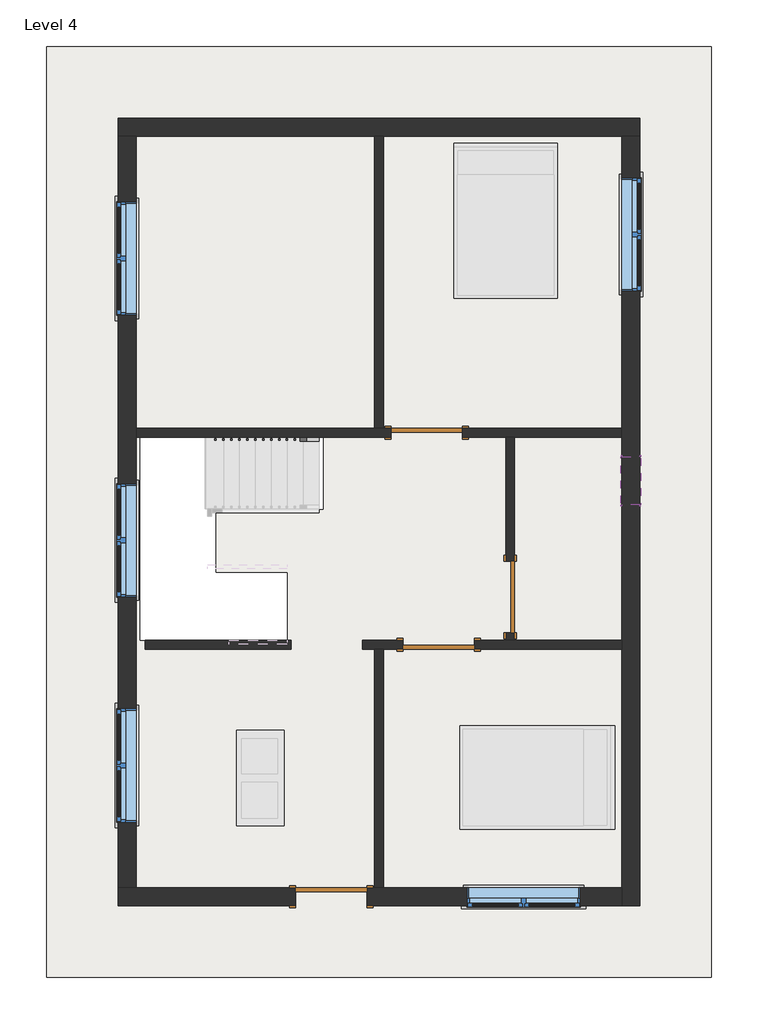
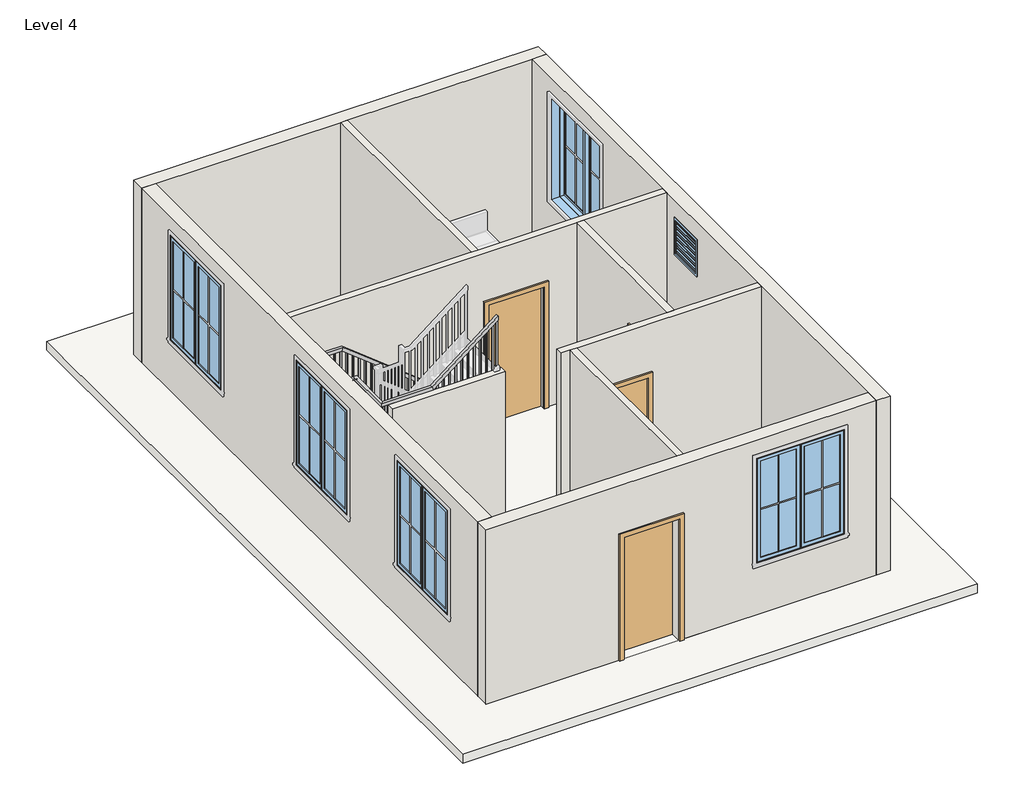
# One storey, part 1 of 2: 10 walls, 6 windows, 4 doors, 1 railing, 1 roof, 1 slab.
"""IFC4 building model written with IfcOpenShell, lengths in millimetres."""

from ifc_helpers import new_model, si_unit, frame, origin, place, context, project, spatial, polyline, outline, extrude, faceted_brep, transform, mapped, element, save
from components import door_e5f9f3c4, door_0ca8825f, window_9ac97e1a, window_f2d8fef0

model = new_model("IFC4")

# Units and contexts
model_context = context("Model", 3, world=origin())
ifc_project = project(units=[si_unit("LENGTHUNIT", "METRE", prefix="MILLI")], contexts=[model_context])

# Site, building, storey
site = spatial("IfcSite", under=ifc_project)
building = spatial("IfcBuilding", under=site)
storey = spatial("IfcBuildingStorey", under=building, Name="Level 4", Elevation=6400.8)

# Doors
placement = place(None, origin())
door_shape = door_e5f9f3c4(model_context)
element("IfcDoor", 1, ObjectType="Single-Flush : 36\" x 84\"", at=placement, inside=storey, context=model_context, shape_type="MappedRepresentation", body=[
    mapped(door_shape, transform((-2225.1840247, 979.1819954, 6400.8), x_axis=(1.0, 0.0, 0.0), y_axis=(0.0, 1.0, 0.0), z_axis=(0.0, 0.0, 1.0))),
])
element("IfcDoor", 2, ObjectType="Single-Flush : 36\" x 84\"", at=placement, inside=storey, context=model_context, shape_type="MappedRepresentation", body=[
    mapped(door_shape, transform((-1158.3840247, -1116.3180046, 6400.8), x_axis=(0.0, -1.0, 0.0), y_axis=(1.0, 0.0, 0.0), z_axis=(0.0, 0.0, 1.0))),
])
element("IfcDoor", 3, ObjectType="Single-Flush : 36\" x 84\"", at=placement, inside=storey, context=model_context, shape_type="MappedRepresentation", body=[
    mapped(door_shape, transform((-2072.7840247, -1725.9180046, 6400.8), x_axis=(-1.0, 0.0, 0.0), y_axis=(0.0, -1.0, 0.0), z_axis=(0.0, 0.0, 1.0))),
])
door_2_shape = door_0ca8825f(model_context)
element("IfcDoor", 4, ObjectType="Single-Flush : 36\" x 84\"", at=placement, inside=storey, context=model_context, shape_type="MappedRepresentation", body=[
    mapped(door_2_shape, transform((-3444.3840247, -4945.3680046, 6400.8), x_axis=(1.0, 0.0, 0.0), y_axis=(0.0, 1.0, 0.0), z_axis=(0.0, 0.0, 1.0))),
])

# Railing
element("IfcRailing", 5, ObjectType="Handrail - Rectangular", at=placement, inside=storey, context=model_context, shape_type="SolidModel", body=[
    faceted_brep([(-3603.1340247, 871.2319954, 7475.6210526), (-3603.1340247, 871.2319954, 7410.8980109), (-3603.1340247, 922.0319954, 7410.8980109), (-3603.1340247, 922.0319954, 7475.6210526), (-5097.5006913, 871.2319954, 8655.3842105), (-5115.1365442, 871.2319954, 8604.5842105), (-5115.1365442, 922.0319954, 8604.5842105), (-5097.5006913, 922.0319954, 8655.3842105), (-5889.1340247, 871.2319954, 8655.3842105), (-5889.1340247, 871.2319954, 8604.5842105), (-5939.9340247, 922.0319954, 8604.5842105), (-5939.9340247, 922.0319954, 8655.3842105), (-5889.1340247, 130.6632454, 8655.3842105), (-5889.1340247, 112.1228815, 8604.5842105), (-5939.9340247, 112.1228815, 8604.5842105), (-5939.9340247, 130.6632454, 8655.3842105), (-5889.1340247, -877.3992546, 9504.2789474), (-5889.1340247, -895.9396185, 9453.4789474), (-5939.9340247, -895.9396185, 9453.4789474), (-5939.9340247, -877.3992546, 9504.2789474), (-5889.1340247, -1617.9680046, 9504.2789474), (-5889.1340247, -1617.9680046, 9453.4789474), (-5939.9340247, -1668.7680046, 9453.4789474), (-5939.9340247, -1668.7680046, 9504.2789474), (-5097.5006913, -1617.9680046, 9504.2789474), (-5079.8648385, -1617.9680046, 9453.4789474), (-5079.8648385, -1668.7680046, 9453.4789474), (-5097.5006913, -1668.7680046, 9504.2789474), (-4009.5340247, -1617.9680046, 10363.2), (-4009.5340247, -1668.7680046, 10363.2), (-4009.5340247, -1668.7680046, 10298.4769583), (-4009.5340247, -1617.9680046, 10298.4769583)], [[[0, 1, 2, 3]], [[1, 0, 4, 5]], [[2, 1, 5, 6]], [[3, 2, 6, 7]], [[0, 3, 7, 4]], [[5, 4, 8, 9]], [[6, 5, 9, 10]], [[7, 6, 10, 11]], [[4, 7, 11, 8]], [[9, 8, 12, 13]], [[10, 9, 13, 14]], [[11, 10, 14, 15]], [[8, 11, 15, 12]], [[13, 12, 16, 17]], [[14, 13, 17, 18]], [[15, 14, 18, 19]], [[12, 15, 19, 16]], [[17, 16, 20, 21]], [[18, 17, 21, 22]], [[19, 18, 22, 23]], [[16, 19, 23, 20]], [[21, 20, 24, 25]], [[22, 21, 25, 26]], [[23, 22, 26, 27]], [[20, 23, 27, 24]], [[28, 29, 30, 31]], [[25, 24, 28, 31]], [[26, 25, 31, 30]], [[27, 26, 30, 29]], [[24, 27, 29, 28]]]),
    extrude(outline(polyline([(10245.8388004, -4076.2090247), (10230.7993267, -4095.2590247), (9288.3789474, -4095.2590247), (9288.3789474, -4076.2090247), (10245.8388004, -4076.2090247)])), frame((0.0, -1652.8930046, 0.0), z_axis=(0.0, 1.0, 0.0), x_axis=(0.0, 0.0, 1.0)), (0.0, 0.0, 1.0), 19.05),
    extrude(outline(polyline([(10165.628274, -4177.8090247), (10150.5888004, -4196.8590247), (9288.3789474, -4196.8590247), (9288.3789474, -4177.8090247), (10165.628274, -4177.8090247)])), frame((0.0, -1652.8930046, 0.0), z_axis=(0.0, 1.0, 0.0), x_axis=(0.0, 0.0, 1.0)), (0.0, 0.0, 1.0), 19.05),
    extrude(outline(polyline([(10085.4177477, -4279.4090247), (10070.378274, -4298.4590247), (9127.9578947, -4298.4590247), (9127.9578947, -4279.4090247), (10085.4177477, -4279.4090247)])), frame((0.0, -1652.8930046, 0.0), z_axis=(0.0, 1.0, 0.0), x_axis=(0.0, 0.0, 1.0)), (0.0, 0.0, 1.0), 19.05),
    extrude(outline(polyline([(10005.2072214, -4381.0090247), (9990.1677477, -4400.0590247), (9127.9578947, -4400.0590247), (9127.9578947, -4381.0090247), (10005.2072214, -4381.0090247)])), frame((0.0, -1652.8930046, 0.0), z_axis=(0.0, 1.0, 0.0), x_axis=(0.0, 0.0, 1.0)), (0.0, 0.0, 1.0), 19.05),
    extrude(outline(polyline([(9924.9966951, -4482.6090247), (9909.9572214, -4501.6590247), (8967.5368421, -4501.6590247), (8967.5368421, -4482.6090247), (9924.9966951, -4482.6090247)])), frame((0.0, -1652.8930046, 0.0), z_axis=(0.0, 1.0, 0.0), x_axis=(0.0, 0.0, 1.0)), (0.0, 0.0, 1.0), 19.05),
    extrude(outline(polyline([(9844.7861688, -4584.2090247), (9829.7466951, -4603.2590247), (8967.5368421, -4603.2590247), (8967.5368421, -4584.2090247), (9844.7861688, -4584.2090247)])), frame((0.0, -1652.8930046, 0.0), z_axis=(0.0, 1.0, 0.0), x_axis=(0.0, 0.0, 1.0)), (0.0, 0.0, 1.0), 19.05),
    extrude(outline(polyline([(9764.5756425, -4685.8090247), (9749.5361688, -4704.8590247), (8807.1157895, -4704.8590247), (8807.1157895, -4685.8090247), (9764.5756425, -4685.8090247)])), frame((0.0, -1652.8930046, 0.0), z_axis=(0.0, 1.0, 0.0), x_axis=(0.0, 0.0, 1.0)), (0.0, 0.0, 1.0), 19.05),
    extrude(outline(polyline([(9684.3651161, -4787.4090247), (9669.3256425, -4806.4590247), (8807.1157895, -4806.4590247), (8807.1157895, -4787.4090247), (9684.3651161, -4787.4090247)])), frame((0.0, -1652.8930046, 0.0), z_axis=(0.0, 1.0, 0.0), x_axis=(0.0, 0.0, 1.0)), (0.0, 0.0, 1.0), 19.05),
    extrude(outline(polyline([(9604.1545898, -4889.0090247), (9589.1151161, -4908.0590247), (8646.6947368, -4908.0590247), (8646.6947368, -4889.0090247), (9604.1545898, -4889.0090247)])), frame((0.0, -1652.8930046, 0.0), z_axis=(0.0, 1.0, 0.0), x_axis=(0.0, 0.0, 1.0)), (0.0, 0.0, 1.0), 19.05),
    extrude(outline(polyline([(9523.9440635, -4990.6090247), (9508.9045898, -5009.6590247), (8646.6947368, -5009.6590247), (8646.6947368, -4990.6090247), (9523.9440635, -4990.6090247)])), frame((0.0, -1652.8930046, 0.0), z_axis=(0.0, 1.0, 0.0), x_axis=(0.0, 0.0, 1.0)), (0.0, 0.0, 1.0), 19.05),
    extrude(outline(polyline([(-5111.2590247, -1652.8930046), (-5111.2590247, -1633.8430046), (-5092.2090247, -1633.8430046), (-5092.2090247, -1652.8930046), (-5111.2590247, -1652.8930046)])), frame((0.0, 0.0, 8486.2736842), z_axis=(0.0, 0.0, 1.0), x_axis=(1.0, 0.0, 0.0)), (0.0, 0.0, 1.0), 967.2052632),
    extrude(outline(polyline([(-5212.8590247, -1652.8930046), (-5212.8590247, -1633.8430046), (-5193.8090247, -1633.8430046), (-5193.8090247, -1652.8930046), (-5212.8590247, -1652.8930046)])), frame((0.0, 0.0, 8486.2736842), z_axis=(0.0, 0.0, 1.0), x_axis=(1.0, 0.0, 0.0)), (0.0, 0.0, 1.0), 967.2052632),
    extrude(outline(polyline([(-5314.4590247, -1652.8930046), (-5314.4590247, -1633.8430046), (-5295.4090247, -1633.8430046), (-5295.4090247, -1652.8930046), (-5314.4590247, -1652.8930046)])), frame((0.0, 0.0, 8486.2736842), z_axis=(0.0, 0.0, 1.0), x_axis=(1.0, 0.0, 0.0)), (0.0, 0.0, 1.0), 967.2052632),
    extrude(outline(polyline([(-5416.0590247, -1652.8930046), (-5416.0590247, -1633.8430046), (-5397.0090247, -1633.8430046), (-5397.0090247, -1652.8930046), (-5416.0590247, -1652.8930046)])), frame((0.0, 0.0, 8486.2736842), z_axis=(0.0, 0.0, 1.0), x_axis=(1.0, 0.0, 0.0)), (0.0, 0.0, 1.0), 967.2052632),
    extrude(outline(polyline([(-5517.6590247, -1652.8930046), (-5517.6590247, -1633.8430046), (-5498.6090247, -1633.8430046), (-5498.6090247, -1652.8930046), (-5517.6590247, -1652.8930046)])), frame((0.0, 0.0, 8486.2736842), z_axis=(0.0, 0.0, 1.0), x_axis=(1.0, 0.0, 0.0)), (0.0, 0.0, 1.0), 967.2052632),
    extrude(outline(polyline([(-5619.2590247, -1652.8930046), (-5619.2590247, -1633.8430046), (-5600.2090247, -1633.8430046), (-5600.2090247, -1652.8930046), (-5619.2590247, -1652.8930046)])), frame((0.0, 0.0, 8486.2736842), z_axis=(0.0, 0.0, 1.0), x_axis=(1.0, 0.0, 0.0)), (0.0, 0.0, 1.0), 967.2052632),
    extrude(outline(polyline([(-5720.8590247, -1652.8930046), (-5720.8590247, -1633.8430046), (-5701.8090247, -1633.8430046), (-5701.8090247, -1652.8930046), (-5720.8590247, -1652.8930046)])), frame((0.0, 0.0, 8486.2736842), z_axis=(0.0, 0.0, 1.0), x_axis=(1.0, 0.0, 0.0)), (0.0, 0.0, 1.0), 967.2052632),
    extrude(outline(polyline([(-5822.4590247, -1652.8930046), (-5822.4590247, -1633.8430046), (-5803.4090247, -1633.8430046), (-5803.4090247, -1652.8930046), (-5822.4590247, -1652.8930046)])), frame((0.0, 0.0, 8486.2736842), z_axis=(0.0, 0.0, 1.0), x_axis=(1.0, 0.0, 0.0)), (0.0, 0.0, 1.0), 967.2052632),
    extrude(outline(polyline([(-5924.0590247, -1532.2430046), (-5905.0090247, -1532.2430046), (-5905.0090247, -1551.2930046), (-5924.0590247, -1551.2930046), (-5924.0590247, -1532.2430046)])), frame((0.0, 0.0, 8486.2736842), z_axis=(0.0, 0.0, 1.0), x_axis=(1.0, 0.0, 0.0)), (0.0, 0.0, 1.0), 967.2052632),
    extrude(outline(polyline([(-5924.0590247, -1430.6430046), (-5905.0090247, -1430.6430046), (-5905.0090247, -1449.6930046), (-5924.0590247, -1449.6930046), (-5924.0590247, -1430.6430046)])), frame((0.0, 0.0, 8486.2736842), z_axis=(0.0, 0.0, 1.0), x_axis=(1.0, 0.0, 0.0)), (0.0, 0.0, 1.0), 967.2052632),
    extrude(outline(polyline([(-5924.0590247, -1329.0430046), (-5905.0090247, -1329.0430046), (-5905.0090247, -1348.0930046), (-5924.0590247, -1348.0930046), (-5924.0590247, -1329.0430046)])), frame((0.0, 0.0, 8486.2736842), z_axis=(0.0, 0.0, 1.0), x_axis=(1.0, 0.0, 0.0)), (0.0, 0.0, 1.0), 967.2052632),
    extrude(outline(polyline([(-5924.0590247, -1227.4430046), (-5905.0090247, -1227.4430046), (-5905.0090247, -1246.4930046), (-5924.0590247, -1246.4930046), (-5924.0590247, -1227.4430046)])), frame((0.0, 0.0, 8486.2736842), z_axis=(0.0, 0.0, 1.0), x_axis=(1.0, 0.0, 0.0)), (0.0, 0.0, 1.0), 967.2052632),
    extrude(outline(polyline([(-5924.0590247, -1125.8430046), (-5905.0090247, -1125.8430046), (-5905.0090247, -1144.8930046), (-5924.0590247, -1144.8930046), (-5924.0590247, -1125.8430046)])), frame((0.0, 0.0, 8486.2736842), z_axis=(0.0, 0.0, 1.0), x_axis=(1.0, 0.0, 0.0)), (0.0, 0.0, 1.0), 967.2052632),
    extrude(outline(polyline([(-5924.0590247, -1024.2430046), (-5905.0090247, -1024.2430046), (-5905.0090247, -1043.2930046), (-5924.0590247, -1043.2930046), (-5924.0590247, -1024.2430046)])), frame((0.0, 0.0, 8486.2736842), z_axis=(0.0, 0.0, 1.0), x_axis=(1.0, 0.0, 0.0)), (0.0, 0.0, 1.0), 967.2052632),
    extrude(outline(polyline([(-5924.0590247, -922.6430046), (-5905.0090247, -922.6430046), (-5905.0090247, -941.6930046), (-5924.0590247, -941.6930046), (-5924.0590247, -922.6430046)])), frame((0.0, 0.0, 8486.2736842), z_axis=(0.0, 0.0, 1.0), x_axis=(1.0, 0.0, 0.0)), (0.0, 0.0, 1.0), 967.2052632),
    extrude(outline(polyline([(-840.0930046, 9406.4502199), (-821.0430046, 9390.4081146), (-821.0430046, 8486.2736842), (-840.0930046, 8486.2736842), (-840.0930046, 9406.4502199)])), frame((-5924.0590247, 0.0, 0.0), z_axis=(1.0, 0.0, 0.0), x_axis=(0.0, 1.0, 0.0)), (0.0, 0.0, 1.0), 19.05),
    extrude(outline(polyline([(-738.4930046, 9320.8923251), (-719.4430046, 9304.8502199), (-719.4430046, 8325.8526316), (-738.4930046, 8325.8526316), (-738.4930046, 9320.8923251)])), frame((-5924.0590247, 0.0, 0.0), z_axis=(1.0, 0.0, 0.0), x_axis=(0.0, 1.0, 0.0)), (0.0, 0.0, 1.0), 19.05),
    extrude(outline(polyline([(-636.8930046, 9235.3344304), (-617.8430046, 9219.2923251), (-617.8430046, 8325.8526316), (-636.8930046, 8325.8526316), (-636.8930046, 9235.3344304)])), frame((-5924.0590247, 0.0, 0.0), z_axis=(1.0, 0.0, 0.0), x_axis=(0.0, 1.0, 0.0)), (0.0, 0.0, 1.0), 19.05),
    extrude(outline(polyline([(-535.2930046, 9149.7765357), (-516.2430046, 9133.7344304), (-516.2430046, 8165.4315789), (-535.2930046, 8165.4315789), (-535.2930046, 9149.7765357)])), frame((-5924.0590247, 0.0, 0.0), z_axis=(1.0, 0.0, 0.0), x_axis=(0.0, 1.0, 0.0)), (0.0, 0.0, 1.0), 19.05),
    extrude(outline(polyline([(-433.6930046, 9064.2186409), (-414.6430046, 9048.1765357), (-414.6430046, 8165.4315789), (-433.6930046, 8165.4315789), (-433.6930046, 9064.2186409)])), frame((-5924.0590247, 0.0, 0.0), z_axis=(1.0, 0.0, 0.0), x_axis=(0.0, 1.0, 0.0)), (0.0, 0.0, 1.0), 19.05),
    extrude(outline(polyline([(-332.0930046, 8978.6607462), (-313.0430046, 8962.6186409), (-313.0430046, 8005.0105263), (-332.0930046, 8005.0105263), (-332.0930046, 8978.6607462)])), frame((-5924.0590247, 0.0, 0.0), z_axis=(1.0, 0.0, 0.0), x_axis=(0.0, 1.0, 0.0)), (0.0, 0.0, 1.0), 19.05),
    extrude(outline(polyline([(-230.4930046, 8893.1028514), (-211.4430046, 8877.0607462), (-211.4430046, 8005.0105263), (-230.4930046, 8005.0105263), (-230.4930046, 8893.1028514)])), frame((-5924.0590247, 0.0, 0.0), z_axis=(1.0, 0.0, 0.0), x_axis=(0.0, 1.0, 0.0)), (0.0, 0.0, 1.0), 19.05),
    extrude(outline(polyline([(-128.8930046, 8807.5449567), (-109.8430046, 8791.5028514), (-109.8430046, 7844.5894737), (-128.8930046, 7844.5894737), (-128.8930046, 8807.5449567)])), frame((-5924.0590247, 0.0, 0.0), z_axis=(1.0, 0.0, 0.0), x_axis=(0.0, 1.0, 0.0)), (0.0, 0.0, 1.0), 19.05),
    extrude(outline(polyline([(-27.2930046, 8721.987062), (-8.2430046, 8705.9449567), (-8.2430046, 7844.5894737), (-27.2930046, 7844.5894737), (-27.2930046, 8721.987062)])), frame((-5924.0590247, 0.0, 0.0), z_axis=(1.0, 0.0, 0.0), x_axis=(0.0, 1.0, 0.0)), (0.0, 0.0, 1.0), 19.05),
    extrude(outline(polyline([(74.3069954, 8636.4291672), (93.3569954, 8620.387062), (93.3569954, 7684.1684211), (74.3069954, 7684.1684211), (74.3069954, 8636.4291672)])), frame((-5924.0590247, 0.0, 0.0), z_axis=(1.0, 0.0, 0.0), x_axis=(0.0, 1.0, 0.0)), (0.0, 0.0, 1.0), 19.05),
    extrude(outline(polyline([(-5924.0590247, 194.9569954), (-5905.0090247, 194.9569954), (-5905.0090247, 175.9069954), (-5924.0590247, 175.9069954), (-5924.0590247, 194.9569954)])), frame((0.0, 0.0, 7684.1684211), z_axis=(0.0, 0.0, 1.0), x_axis=(1.0, 0.0, 0.0)), (0.0, 0.0, 1.0), 920.4157895),
    extrude(outline(polyline([(-5924.0590247, 296.5569954), (-5905.0090247, 296.5569954), (-5905.0090247, 277.5069954), (-5924.0590247, 277.5069954), (-5924.0590247, 296.5569954)])), frame((0.0, 0.0, 7684.1684211), z_axis=(0.0, 0.0, 1.0), x_axis=(1.0, 0.0, 0.0)), (0.0, 0.0, 1.0), 920.4157895),
    extrude(outline(polyline([(-5924.0590247, 398.1569954), (-5905.0090247, 398.1569954), (-5905.0090247, 379.1069954), (-5924.0590247, 379.1069954), (-5924.0590247, 398.1569954)])), frame((0.0, 0.0, 7684.1684211), z_axis=(0.0, 0.0, 1.0), x_axis=(1.0, 0.0, 0.0)), (0.0, 0.0, 1.0), 920.4157895),
    extrude(outline(polyline([(-5924.0590247, 499.7569954), (-5905.0090247, 499.7569954), (-5905.0090247, 480.7069954), (-5924.0590247, 480.7069954), (-5924.0590247, 499.7569954)])), frame((0.0, 0.0, 7684.1684211), z_axis=(0.0, 0.0, 1.0), x_axis=(1.0, 0.0, 0.0)), (0.0, 0.0, 1.0), 920.4157895),
    extrude(outline(polyline([(-5924.0590247, 601.3569954), (-5905.0090247, 601.3569954), (-5905.0090247, 582.3069954), (-5924.0590247, 582.3069954), (-5924.0590247, 601.3569954)])), frame((0.0, 0.0, 7684.1684211), z_axis=(0.0, 0.0, 1.0), x_axis=(1.0, 0.0, 0.0)), (0.0, 0.0, 1.0), 920.4157895),
    extrude(outline(polyline([(-5924.0590247, 702.9569954), (-5905.0090247, 702.9569954), (-5905.0090247, 683.9069954), (-5924.0590247, 683.9069954), (-5924.0590247, 702.9569954)])), frame((0.0, 0.0, 7684.1684211), z_axis=(0.0, 0.0, 1.0), x_axis=(1.0, 0.0, 0.0)), (0.0, 0.0, 1.0), 920.4157895),
    extrude(outline(polyline([(-5924.0590247, 804.5569954), (-5905.0090247, 804.5569954), (-5905.0090247, 785.5069954), (-5924.0590247, 785.5069954), (-5924.0590247, 804.5569954)])), frame((0.0, 0.0, 7684.1684211), z_axis=(0.0, 0.0, 1.0), x_axis=(1.0, 0.0, 0.0)), (0.0, 0.0, 1.0), 920.4157895),
    extrude(outline(polyline([(-5828.8090247, 906.1569954), (-5828.8090247, 887.1069954), (-5847.8590247, 887.1069954), (-5847.8590247, 906.1569954), (-5828.8090247, 906.1569954)])), frame((0.0, 0.0, 7684.1684211), z_axis=(0.0, 0.0, 1.0), x_axis=(1.0, 0.0, 0.0)), (0.0, 0.0, 1.0), 920.4157895),
    extrude(outline(polyline([(-5727.2090247, 906.1569954), (-5727.2090247, 887.1069954), (-5746.2590247, 887.1069954), (-5746.2590247, 906.1569954), (-5727.2090247, 906.1569954)])), frame((0.0, 0.0, 7684.1684211), z_axis=(0.0, 0.0, 1.0), x_axis=(1.0, 0.0, 0.0)), (0.0, 0.0, 1.0), 920.4157895),
    extrude(outline(polyline([(-5625.6090247, 906.1569954), (-5625.6090247, 887.1069954), (-5644.6590247, 887.1069954), (-5644.6590247, 906.1569954), (-5625.6090247, 906.1569954)])), frame((0.0, 0.0, 7684.1684211), z_axis=(0.0, 0.0, 1.0), x_axis=(1.0, 0.0, 0.0)), (0.0, 0.0, 1.0), 920.4157895),
    extrude(outline(polyline([(-5524.0090247, 906.1569954), (-5524.0090247, 887.1069954), (-5543.0590247, 887.1069954), (-5543.0590247, 906.1569954), (-5524.0090247, 906.1569954)])), frame((0.0, 0.0, 7684.1684211), z_axis=(0.0, 0.0, 1.0), x_axis=(1.0, 0.0, 0.0)), (0.0, 0.0, 1.0), 920.4157895),
    extrude(outline(polyline([(-5422.4090247, 906.1569954), (-5422.4090247, 887.1069954), (-5441.4590247, 887.1069954), (-5441.4590247, 906.1569954), (-5422.4090247, 906.1569954)])), frame((0.0, 0.0, 7684.1684211), z_axis=(0.0, 0.0, 1.0), x_axis=(1.0, 0.0, 0.0)), (0.0, 0.0, 1.0), 920.4157895),
    extrude(outline(polyline([(-5320.8090247, 906.1569954), (-5320.8090247, 887.1069954), (-5339.8590247, 887.1069954), (-5339.8590247, 906.1569954), (-5320.8090247, 906.1569954)])), frame((0.0, 0.0, 7684.1684211), z_axis=(0.0, 0.0, 1.0), x_axis=(1.0, 0.0, 0.0)), (0.0, 0.0, 1.0), 920.4157895),
    extrude(outline(polyline([(-5219.2090247, 906.1569954), (-5219.2090247, 887.1069954), (-5238.2590247, 887.1069954), (-5238.2590247, 906.1569954), (-5219.2090247, 906.1569954)])), frame((0.0, 0.0, 7684.1684211), z_axis=(0.0, 0.0, 1.0), x_axis=(1.0, 0.0, 0.0)), (0.0, 0.0, 1.0), 920.4157895),
    extrude(outline(polyline([(-5117.6090247, 906.1569954), (-5117.6090247, 887.1069954), (-5136.6590247, 887.1069954), (-5136.6590247, 906.1569954), (-5117.6090247, 906.1569954)])), frame((0.0, 0.0, 7684.1684211), z_axis=(0.0, 0.0, 1.0), x_axis=(1.0, 0.0, 0.0)), (0.0, 0.0, 1.0), 920.4157895),
    extrude(outline(polyline([(8526.3256425, -5016.0090247), (8541.3651161, -5035.0590247), (7684.1684211, -5035.0590247), (7684.1684211, -5016.0090247), (8526.3256425, -5016.0090247)])), frame((0.0, 887.1069954, 0.0), z_axis=(0.0, 1.0, 0.0), x_axis=(0.0, 0.0, 1.0)), (0.0, 0.0, 1.0), 19.05),
    extrude(outline(polyline([(8446.1151161, -4914.4090247), (8461.1545898, -4933.4590247), (7523.7473684, -4933.4590247), (7523.7473684, -4914.4090247), (8446.1151161, -4914.4090247)])), frame((0.0, 887.1069954, 0.0), z_axis=(0.0, 1.0, 0.0), x_axis=(0.0, 0.0, 1.0)), (0.0, 0.0, 1.0), 19.05),
    extrude(outline(polyline([(8365.9045898, -4812.8090247), (8380.9440635, -4831.8590247), (7523.7473684, -4831.8590247), (7523.7473684, -4812.8090247), (8365.9045898, -4812.8090247)])), frame((0.0, 887.1069954, 0.0), z_axis=(0.0, 1.0, 0.0), x_axis=(0.0, 0.0, 1.0)), (0.0, 0.0, 1.0), 19.05),
    extrude(outline(polyline([(8285.6940635, -4711.2090247), (8300.7335372, -4730.2590247), (7363.3263158, -4730.2590247), (7363.3263158, -4711.2090247), (8285.6940635, -4711.2090247)])), frame((0.0, 887.1069954, 0.0), z_axis=(0.0, 1.0, 0.0), x_axis=(0.0, 0.0, 1.0)), (0.0, 0.0, 1.0), 19.05),
    extrude(outline(polyline([(8205.4835372, -4609.6090247), (8220.5230109, -4628.6590247), (7363.3263158, -4628.6590247), (7363.3263158, -4609.6090247), (8205.4835372, -4609.6090247)])), frame((0.0, 887.1069954, 0.0), z_axis=(0.0, 1.0, 0.0), x_axis=(0.0, 0.0, 1.0)), (0.0, 0.0, 1.0), 19.05),
    extrude(outline(polyline([(8125.2730109, -4508.0090247), (8140.3124846, -4527.0590247), (7202.9052632, -4527.0590247), (7202.9052632, -4508.0090247), (8125.2730109, -4508.0090247)])), frame((0.0, 887.1069954, 0.0), z_axis=(0.0, 1.0, 0.0), x_axis=(0.0, 0.0, 1.0)), (0.0, 0.0, 1.0), 19.05),
    extrude(outline(polyline([(8045.0624846, -4406.4090247), (8060.1019583, -4425.4590247), (7202.9052632, -4425.4590247), (7202.9052632, -4406.4090247), (8045.0624846, -4406.4090247)])), frame((0.0, 887.1069954, 0.0), z_axis=(0.0, 1.0, 0.0), x_axis=(0.0, 0.0, 1.0)), (0.0, 0.0, 1.0), 19.05),
    extrude(outline(polyline([(7964.8519583, -4304.8090247), (7979.8914319, -4323.8590247), (7042.4842105, -4323.8590247), (7042.4842105, -4304.8090247), (7964.8519583, -4304.8090247)])), frame((0.0, 887.1069954, 0.0), z_axis=(0.0, 1.0, 0.0), x_axis=(0.0, 0.0, 1.0)), (0.0, 0.0, 1.0), 19.05),
    extrude(outline(polyline([(7884.6414319, -4203.2090247), (7899.6809056, -4222.2590247), (7042.4842105, -4222.2590247), (7042.4842105, -4203.2090247), (7884.6414319, -4203.2090247)])), frame((0.0, 887.1069954, 0.0), z_axis=(0.0, 1.0, 0.0), x_axis=(0.0, 0.0, 1.0)), (0.0, 0.0, 1.0), 19.05),
    extrude(outline(polyline([(7804.4309056, -4101.6090247), (7819.4703793, -4120.6590247), (6882.0631579, -4120.6590247), (6882.0631579, -4101.6090247), (7804.4309056, -4101.6090247)])), frame((0.0, 887.1069954, 0.0), z_axis=(0.0, 1.0, 0.0), x_axis=(0.0, 0.0, 1.0)), (0.0, 0.0, 1.0), 19.05),
    extrude(outline(polyline([(7724.2203793, -4000.0090247), (7739.259853, -4019.0590247), (6882.0631579, -4019.0590247), (6882.0631579, -4000.0090247), (7724.2203793, -4000.0090247)])), frame((0.0, 887.1069954, 0.0), z_axis=(0.0, 1.0, 0.0), x_axis=(0.0, 0.0, 1.0)), (0.0, 0.0, 1.0), 19.05),
    extrude(outline(polyline([(7644.009853, -3898.4090247), (7659.0493267, -3917.4590247), (6721.6421053, -3917.4590247), (6721.6421053, -3898.4090247), (7644.009853, -3898.4090247)])), frame((0.0, 887.1069954, 0.0), z_axis=(0.0, 1.0, 0.0), x_axis=(0.0, 0.0, 1.0)), (0.0, 0.0, 1.0), 19.05),
    extrude(outline(polyline([(7563.7993267, -3796.8090247), (7578.8388004, -3815.8590247), (6721.6421053, -3815.8590247), (6721.6421053, -3796.8090247), (7563.7993267, -3796.8090247)])), frame((0.0, 887.1069954, 0.0), z_axis=(0.0, 1.0, 0.0), x_axis=(0.0, 0.0, 1.0)), (0.0, 0.0, 1.0), 19.05),
    extrude(outline(polyline([(7483.5888004, -3695.2090247), (7498.628274, -3714.2590247), (6561.2210526, -3714.2590247), (6561.2210526, -3695.2090247), (7483.5888004, -3695.2090247)])), frame((0.0, 887.1069954, 0.0), z_axis=(0.0, 1.0, 0.0), x_axis=(0.0, 0.0, 1.0)), (0.0, 0.0, 1.0), 19.05),
    extrude(outline(polyline([(-5924.0590247, -1633.8430046), (-5905.0090247, -1633.8430046), (-5905.0090247, -1652.8930046), (-5924.0590247, -1652.8930046), (-5924.0590247, -1633.8430046)])), frame((0.0, 0.0, 8486.2736842), z_axis=(0.0, 0.0, 1.0), x_axis=(1.0, 0.0, 0.0)), (0.0, 0.0, 1.0), 967.2052632),
    extrude(outline(polyline([(-5905.0090247, 906.1569954), (-5905.0090247, 887.1069954), (-5924.0590247, 887.1069954), (-5924.0590247, 906.1569954), (-5905.0090247, 906.1569954)])), frame((0.0, 0.0, 7684.1684211), z_axis=(0.0, 0.0, 1.0), x_axis=(1.0, 0.0, 0.0)), (0.0, 0.0, 1.0), 920.4157895),
    extrude(outline(polyline([(10298.4769583, -4009.5340247), (10283.4374846, -4028.5840247), (9288.3789474, -4028.5840247), (9288.3789474, -4009.5340247), (10298.4769583, -4009.5340247)])), frame((0.0, -1652.8930046, 0.0), z_axis=(0.0, 1.0, 0.0), x_axis=(0.0, 0.0, 1.0)), (0.0, 0.0, 1.0), 19.05),
    extrude(outline(polyline([(7410.8980109, -3603.1340247), (7425.9374846, -3622.1840247), (6561.2210526, -3622.1840247), (6561.2210526, -3603.1340247), (7410.8980109, -3603.1340247)])), frame((0.0, 887.1069954, 0.0), z_axis=(0.0, 1.0, 0.0), x_axis=(0.0, 0.0, 1.0)), (0.0, 0.0, 1.0), 19.05),
])

# Roof
element("IfcRoof", 6, ObjectType="ROOF 6\"", at=placement, inside=storey, context=model_context, shape_type="SweptSolid", body=[
    extrude(outline(polyline([(-7082.9340247, 5913.1319954), (1413.3659753, 5913.1319954), (1413.3659753, -5974.0680046), (-7082.9340247, -5974.0680046), (-7082.9340247, 5913.1319954)]), holes=[polyline([(-5889.1340247, 922.0319954), (-5889.1340247, -1668.7680046), (-4009.5340247, -1668.7680046), (-4009.5340247, -805.1680046), (-4923.9340247, -805.1680046), (-4923.9340247, 7.6319954), (-3552.3340247, 7.6319954), (-3552.3340247, 922.0319954), (-5889.1340247, 922.0319954)])]), frame((0.0, 0.0, 6248.4), z_axis=(0.0, 0.0, 1.0), x_axis=(1.0, 0.0, 0.0)), (0.0, 0.0, 1.0), 152.4),
])

# Slab
element("IfcSlab", 7, ObjectType="FLOOR 6\"", at=placement, inside=storey, context=model_context, shape_type="SweptSolid", body=[
    extrude(outline(polyline([(498.9659753, 4998.7319954), (498.9659753, -5059.6680046), (-6168.5340247, -5059.6680046), (-6168.5340247, 4998.7319954), (498.9659753, 4998.7319954)]), holes=[polyline([(-5889.1340247, 922.0319954), (-5889.1340247, -1668.7680046), (-4009.5340247, -1668.7680046), (-4009.5340247, -805.1680046), (-4923.9340247, -805.1680046), (-4923.9340247, 7.6319954), (-3552.3340247, 7.6319954), (-3552.3340247, 922.0319954), (-5889.1340247, 922.0319954)])]), frame((0.0, 0.0, 6248.4), z_axis=(0.0, 0.0, 1.0), x_axis=(1.0, 0.0, 0.0)), (0.0, 0.0, 1.0), 152.4),
])

# Walls
element("IfcWall", 8, ObjectType="WALL 4.5\"", at=placement, inside=storey, context=model_context, shape_type="SweptSolid", body=[
    extrude(outline(polyline([(-2891.9340247, 1036.3319954), (-2891.9340247, 4770.1319954), (-2777.6340247, 4770.1319954), (-2777.6340247, 1036.3319954), (-2891.9340247, 1036.3319954)])), frame((0.0, 0.0, 6400.8), z_axis=(0.0, 0.0, 1.0), x_axis=(1.0, 0.0, 0.0)), (0.0, 0.0, 1.0), 3048.0),
])
element("IfcWall", 9, ObjectType="WALL 4.5\"", at=placement, inside=storey, context=model_context, shape_type="Brep", body=[
    faceted_brep([(-1767.9840247, 922.0319954, 8534.4), (-1767.9840247, 922.0319954, 6400.8), (-1215.5340247, 922.0319954, 6400.8), (-1101.2340247, 922.0319954, 6400.8), (270.3659753, 922.0319954, 6400.8), (270.3659753, 922.0319954, 9448.8), (-1101.2340247, 922.0319954, 9448.8), (-1215.5340247, 922.0319954, 9448.8), (-3552.3340247, 922.0319954, 9448.8), (-5889.1340247, 922.0319954, 9448.8), (-5939.9340247, 922.0319954, 9448.8), (-5939.9340247, 922.0319954, 6400.8), (-2682.3840247, 922.0319954, 6400.8), (-2682.3840247, 922.0319954, 8534.4), (270.3659753, 1036.3319954, 6400.8), (-1767.9840247, 1036.3319954, 6400.8), (-1767.9840247, 1036.3319954, 8534.4), (-2682.3840247, 1036.3319954, 8534.4), (-2682.3840247, 1036.3319954, 6400.8), (-2777.6340247, 1036.3319954, 6400.8), (-2891.9340247, 1036.3319954, 6400.8), (-5939.9340247, 1036.3319954, 6400.8), (-5939.9340247, 1036.3319954, 9448.8), (-2891.9340247, 1036.3319954, 9448.8), (-2777.6340247, 1036.3319954, 9448.8), (270.3659753, 1036.3319954, 9448.8)], [[[0, 1, 2, 3, 4, 5, 6, 7, 8, 9, 10, 11, 12, 13]], [[14, 15, 16, 17, 18, 19, 20, 21, 22, 23, 24, 25]], [[12, 11, 21, 20, 19, 18]], [[4, 3, 2, 1, 15, 14]], [[5, 4, 14, 25]], [[11, 10, 22, 21]], [[16, 15, 1, 0]], [[17, 16, 0, 13]], [[18, 17, 13, 12]], [[10, 9, 8, 7, 6, 5, 25, 24, 23, 22]]]),
])
element("IfcWall", 10, ObjectType="WALL 4.5\"", at=placement, inside=storey, context=model_context, shape_type="SweptSolid", body=[
    extrude(outline(polyline([(-1573.5180046, 8534.4), (-1573.5180046, 6400.8), (-1668.7680046, 6400.8), (-1668.7680046, 9448.8), (922.0319954, 9448.8), (922.0319954, 6400.8), (-659.1180046, 6400.8), (-659.1180046, 8534.4), (-1573.5180046, 8534.4)])), frame((-1215.5340247, 0.0, 0.0), z_axis=(1.0, 0.0, 0.0), x_axis=(0.0, 1.0, 0.0)), (0.0, 0.0, 1.0), 114.3),
])
element("IfcWall", 11, ObjectType="WALL 4.5\"", at=placement, inside=storey, context=model_context, shape_type="Brep", body=[
    faceted_brep([(-2529.9840247, -1668.7680046, 8534.4), (-2529.9840247, -1668.7680046, 6400.8), (-3044.3340247, -1668.7680046, 6400.8), (-3044.3340247, -1668.7680046, 9448.8), (-1215.5340247, -1668.7680046, 9448.8), (-1101.2340247, -1668.7680046, 9448.8), (270.3659753, -1668.7680046, 9448.8), (270.3659753, -1668.7680046, 6400.8), (-1101.2340247, -1668.7680046, 6400.8), (-1215.5340247, -1668.7680046, 6400.8), (-1615.5840247, -1668.7680046, 6400.8), (-1615.5840247, -1668.7680046, 8534.4), (-3044.3340247, -1783.0680046, 6400.8), (-2891.9340247, -1783.0680046, 6400.8), (-2777.6340247, -1783.0680046, 6400.8), (-2529.9840247, -1783.0680046, 6400.8), (-2529.9840247, -1783.0680046, 8534.4), (-1615.5840247, -1783.0680046, 8534.4), (-1615.5840247, -1783.0680046, 6400.8), (270.3659753, -1783.0680046, 6400.8), (270.3659753, -1783.0680046, 9448.8), (-2777.6340247, -1783.0680046, 9448.8), (-2891.9340247, -1783.0680046, 9448.8), (-3044.3340247, -1783.0680046, 9448.8)], [[[0, 1, 2, 3, 4, 5, 6, 7, 8, 9, 10, 11]], [[12, 13, 14, 15, 16, 17, 18, 19, 20, 21, 22, 23]], [[2, 1, 15, 14, 13, 12]], [[10, 9, 8, 7, 19, 18]], [[3, 2, 12, 23]], [[7, 6, 20, 19]], [[16, 15, 1, 0]], [[17, 16, 0, 11]], [[18, 17, 11, 10]], [[6, 5, 4, 3, 23, 22, 21, 20]]]),
])
element("IfcWall", 12, ObjectType="WALL 4.5\"", at=placement, inside=storey, context=model_context, shape_type="Brep", body=[
    faceted_brep([(-5825.6340247, -1783.0680046, 6400.8), (-3958.7340247, -1783.0680046, 6400.8), (-3958.7340247, -1783.0680046, 9448.8), (-5825.6340247, -1783.0680046, 9448.8), (-5825.6340247, -1668.7680046, 6400.8), (-5825.6340247, -1668.7680046, 9448.8), (-4009.5340247, -1668.7680046, 9448.8), (-3958.7340247, -1668.7680046, 9448.8), (-3958.7340247, -1668.7680046, 6400.8)], [[[0, 1, 2, 3]], [[4, 5, 6, 7, 8]], [[1, 0, 4, 8]], [[2, 1, 8, 7]], [[0, 3, 5, 4]], [[3, 2, 7, 6, 5]]]),
])
element("IfcWall", 13, ObjectType="WALL 4.5\"", at=placement, inside=storey, context=model_context, shape_type="SweptSolid", body=[
    extrude(outline(polyline([(-2891.9340247, -4831.0680046), (-2891.9340247, -1783.0680046), (-2777.6340247, -1783.0680046), (-2777.6340247, -4831.0680046), (-2891.9340247, -4831.0680046)])), frame((0.0, 0.0, 6400.8), z_axis=(0.0, 0.0, 1.0), x_axis=(1.0, 0.0, 0.0)), (0.0, 0.0, 1.0), 3048.0),
])
element("IfcWall", 14, ObjectType="WALL 9\"", at=placement, inside=storey, context=model_context, shape_type="Brep", body=[
    faceted_brep([(-6168.5340247, 4770.1319954, 6400.8), (-5939.9340247, 4770.1319954, 6400.8), (-2891.9340247, 4770.1319954, 6400.8), (-2777.6340247, 4770.1319954, 6400.8), (270.3659753, 4770.1319954, 6400.8), (498.9659753, 4770.1319954, 6400.8), (498.9659753, 4770.1319954, 9448.8), (270.3659753, 4770.1319954, 9448.8), (-2777.6340247, 4770.1319954, 9448.8), (-2891.9340247, 4770.1319954, 9448.8), (-5939.9340247, 4770.1319954, 9448.8), (-6168.5340247, 4770.1319954, 9448.8), (-6168.5340247, 4998.7319954, 6400.8), (-6168.5340247, 4998.7319954, 9448.8), (498.9659753, 4998.7319954, 9448.8), (498.9659753, 4998.7319954, 6400.8)], [[[0, 1, 2, 3, 4, 5, 6, 7, 8, 9, 10, 11]], [[12, 13, 14, 15]], [[5, 4, 3, 2, 1, 0, 12, 15]], [[6, 5, 15, 14]], [[0, 11, 13, 12]], [[11, 10, 9, 8, 7, 6, 14, 13]]]),
])
element("IfcWall", 15, ObjectType="WALL 9\"", at=placement, inside=storey, context=model_context, shape_type="Brep", body=[
    faceted_brep([(270.3659753, 4770.1319954, 6400.8), (270.3659753, 1036.3319954, 6400.8), (270.3659753, 922.0319954, 6400.8), (270.3659753, -1668.7680046, 6400.8), (270.3659753, -1783.0680046, 6400.8), (270.3659753, -4831.0680046, 6400.8), (270.3659753, -5059.6680046, 6400.8), (270.3659753, -5059.6680046, 9448.8), (270.3659753, -4831.0680046, 9448.8), (270.3659753, -1783.0680046, 9448.8), (270.3659753, -1668.7680046, 9448.8), (270.3659753, 922.0319954, 9448.8), (270.3659753, 1036.3319954, 9448.8), (270.3659753, 4770.1319954, 9448.8), (270.3659753, 2788.9319954, 9144.0), (270.3659753, 2788.9319954, 7315.2), (270.3659753, 4236.7319954, 7315.2), (270.3659753, 4236.7319954, 9144.0), (270.3659753, 64.7819954, 9144.0), (270.3659753, 64.7819954, 8534.4), (270.3659753, 674.3819954, 8534.4), (270.3659753, 674.3819954, 9144.0), (498.9659753, 4770.1319954, 6400.8), (498.9659753, 4770.1319954, 9448.8), (498.9659753, -5059.6680046, 9448.8), (498.9659753, -5059.6680046, 6400.8), (498.9659753, 2788.9319954, 9144.0), (498.9659753, 4236.7319954, 9144.0), (498.9659753, 4236.7319954, 7315.2), (498.9659753, 2788.9319954, 7315.2), (498.9659753, 64.7819954, 9144.0), (498.9659753, 674.3819954, 9144.0), (498.9659753, 674.3819954, 8534.4), (498.9659753, 64.7819954, 8534.4)], [[[0, 1, 2, 3, 4, 5, 6, 7, 8, 9, 10, 11, 12, 13], [14, 15, 16, 17], [18, 19, 20, 21]], [[22, 23, 24, 25], [26, 27, 28, 29], [30, 31, 32, 33]], [[6, 5, 4, 3, 2, 1, 0, 22, 25]], [[0, 13, 23, 22]], [[7, 6, 25, 24]], [[15, 14, 26, 29]], [[16, 15, 29, 28]], [[17, 16, 28, 27]], [[14, 17, 27, 26]], [[19, 18, 30, 33]], [[20, 19, 33, 32]], [[21, 20, 32, 31]], [[18, 21, 31, 30]], [[13, 12, 11, 10, 9, 8, 7, 24, 23]]]),
])
element("IfcWall", 16, ObjectType="WALL 9\"", at=placement, inside=storey, context=model_context, shape_type="Brep", body=[
    faceted_brep([(270.3659753, -4831.0680046, 6400.8), (-2777.6340247, -4831.0680046, 6400.8), (-2891.9340247, -4831.0680046, 6400.8), (-2987.1840247, -4831.0680046, 6400.8), (-2987.1840247, -4831.0680046, 8534.4), (-3901.5840247, -4831.0680046, 8534.4), (-3901.5840247, -4831.0680046, 6400.8), (-5939.9340247, -4831.0680046, 6400.8), (-6168.5340247, -4831.0680046, 6400.8), (-6168.5340247, -4831.0680046, 9448.8), (-5939.9340247, -4831.0680046, 9448.8), (-2891.9340247, -4831.0680046, 9448.8), (-2777.6340247, -4831.0680046, 9448.8), (270.3659753, -4831.0680046, 9448.8), (-1710.8340247, -4831.0680046, 9144.0), (-1710.8340247, -4831.0680046, 7315.2), (-263.0340247, -4831.0680046, 7315.2), (-263.0340247, -4831.0680046, 9144.0), (-2987.1840247, -5059.6680046, 8534.4), (-2987.1840247, -5059.6680046, 6400.8), (270.3659753, -5059.6680046, 6400.8), (270.3659753, -5059.6680046, 9448.8), (-6168.5340247, -5059.6680046, 9448.8), (-6168.5340247, -5059.6680046, 6400.8), (-3901.5840247, -5059.6680046, 6400.8), (-3901.5840247, -5059.6680046, 8534.4), (-1710.8340247, -5059.6680046, 9144.0), (-263.0340247, -5059.6680046, 9144.0), (-263.0340247, -5059.6680046, 7315.2), (-1710.8340247, -5059.6680046, 7315.2)], [[[0, 1, 2, 3, 4, 5, 6, 7, 8, 9, 10, 11, 12, 13], [14, 15, 16, 17]], [[18, 19, 20, 21, 22, 23, 24, 25], [26, 27, 28, 29]], [[24, 23, 8, 7, 6]], [[20, 19, 3, 2, 1, 0]], [[0, 13, 21, 20]], [[9, 8, 23, 22]], [[15, 14, 26, 29]], [[16, 15, 29, 28]], [[17, 16, 28, 27]], [[14, 17, 27, 26]], [[4, 3, 19, 18]], [[5, 4, 18, 25]], [[6, 5, 25, 24]], [[13, 12, 11, 10, 9, 22, 21]]]),
])
element("IfcWall", 17, ObjectType="WALL 9\"", at=placement, inside=storey, context=model_context, shape_type="Brep", body=[
    faceted_brep([(-5939.9340247, -4831.0680046, 6400.8), (-5939.9340247, 922.0319954, 6400.8), (-5939.9340247, 1036.3319954, 6400.8), (-5939.9340247, 4770.1319954, 6400.8), (-5939.9340247, 4770.1319954, 9448.8), (-5939.9340247, 1036.3319954, 9448.8), (-5939.9340247, 922.0319954, 9448.8), (-5939.9340247, -4831.0680046, 9448.8), (-5939.9340247, -2545.0680046, 9144.0), (-5939.9340247, -2545.0680046, 7315.2), (-5939.9340247, -3992.8680046, 7315.2), (-5939.9340247, -3992.8680046, 9144.0), (-5939.9340247, 3931.9319954, 9144.0), (-5939.9340247, 3931.9319954, 7315.2), (-5939.9340247, 2484.1319954, 7315.2), (-5939.9340247, 2484.1319954, 9144.0), (-5939.9340247, 331.4819954, 9144.0), (-5939.9340247, 331.4819954, 7315.2), (-5939.9340247, -1116.3180046, 7315.2), (-5939.9340247, -1116.3180046, 9144.0), (-6168.5340247, -4831.0680046, 6400.8), (-6168.5340247, -4831.0680046, 9448.8), (-6168.5340247, 4770.1319954, 9448.8), (-6168.5340247, 4770.1319954, 6400.8), (-6168.5340247, -2545.0680046, 9144.0), (-6168.5340247, -3992.8680046, 9144.0), (-6168.5340247, -3992.8680046, 7315.2), (-6168.5340247, -2545.0680046, 7315.2), (-6168.5340247, 3931.9319954, 9144.0), (-6168.5340247, 2484.1319954, 9144.0), (-6168.5340247, 2484.1319954, 7315.2), (-6168.5340247, 3931.9319954, 7315.2), (-6168.5340247, 331.4819954, 9144.0), (-6168.5340247, -1116.3180046, 9144.0), (-6168.5340247, -1116.3180046, 7315.2), (-6168.5340247, 331.4819954, 7315.2)], [[[0, 1, 2, 3, 4, 5, 6, 7], [8, 9, 10, 11], [12, 13, 14, 15], [16, 17, 18, 19]], [[20, 21, 22, 23], [24, 25, 26, 27], [28, 29, 30, 31], [32, 33, 34, 35]], [[3, 2, 1, 0, 20, 23]], [[0, 7, 21, 20]], [[4, 3, 23, 22]], [[9, 8, 24, 27]], [[10, 9, 27, 26]], [[11, 10, 26, 25]], [[8, 11, 25, 24]], [[13, 12, 28, 31]], [[14, 13, 31, 30]], [[15, 14, 30, 29]], [[12, 15, 29, 28]], [[17, 16, 32, 35]], [[18, 17, 35, 34]], [[19, 18, 34, 33]], [[16, 19, 33, 32]], [[7, 6, 5, 4, 22, 21]]]),
])

# Windows
window_shape = window_9ac97e1a(model_context)
element("IfcWindow", 18, ObjectType="Window-Casement-Double : 57\" x 72\"", at=placement, inside=storey, context=model_context, shape_type="MappedRepresentation", body=[
    mapped(window_shape, transform((-986.9340247, -4945.3680046, 6400.8), x_axis=(-1.0, 0.0, 0.0), y_axis=(0.0, -1.0, 0.0), z_axis=(0.0, 0.0, 1.0))),
])
element("IfcWindow", 19, ObjectType="Window-Casement-Double : 57\" x 72\"", at=placement, inside=storey, context=model_context, shape_type="MappedRepresentation", body=[
    mapped(window_shape, transform((-6054.2340247, -3268.9680046, 6400.8), x_axis=(0.0, 1.0, 0.0), y_axis=(-1.0, 0.0, 0.0), z_axis=(0.0, 0.0, 1.0))),
])
element("IfcWindow", 20, ObjectType="Window-Casement-Double : 57\" x 72\"", at=placement, inside=storey, context=model_context, shape_type="MappedRepresentation", body=[
    mapped(window_shape, transform((384.6659753, 3512.8319954, 6400.8), x_axis=(0.0, -1.0, 0.0), y_axis=(1.0, 0.0, 0.0), z_axis=(0.0, 0.0, 1.0))),
])
element("IfcWindow", 21, ObjectType="Window-Casement-Double : 57\" x 72\"", at=placement, inside=storey, context=model_context, shape_type="MappedRepresentation", body=[
    mapped(window_shape, transform((-6054.2340247, 3208.0319954, 6400.8), x_axis=(0.0, 1.0, 0.0), y_axis=(-1.0, 0.0, 0.0), z_axis=(0.0, 0.0, 1.0))),
])
element("IfcWindow", 22, ObjectType="Window-Casement-Double : 57\" x 72\"", at=placement, inside=storey, context=model_context, shape_type="MappedRepresentation", body=[
    mapped(window_shape, transform((-6054.2340247, -392.4180046, 6400.8), x_axis=(0.0, 1.0, 0.0), y_axis=(-1.0, 0.0, 0.0), z_axis=(0.0, 0.0, 1.0))),
])
window_2_shape = window_f2d8fef0(model_context)
element("IfcWindow", 23, ObjectType="Window-Louvers : 24\" x 24\"", at=placement, inside=storey, context=model_context, shape_type="MappedRepresentation", body=[
    mapped(window_2_shape, transform((378.3159753, 369.5819954, 7620.0), x_axis=(0.0, 1.0, 0.0), y_axis=(-1.0, 0.0, 0.0), z_axis=(0.0, 0.0, 1.0))),
])

save(model, "model.ifc")

# Revit data of these elements
# Type "Single-Flush : 36\" x 84\""
#   Type Mark = "1"
#   Construction Type Id = "MDOOR"
#   Assembly Code = "C1020"
#   Analytic Construction = "Metal"
#   Thickness = 0' - 2"
#   Heat Transfer Coefficient (U) = 0.651978 BTU/(h·ft²·°F)
#   Height = 7' - 0"
#   Trim Projection Ext = 0' - 1"
#   Trim Projection Int = 0' - 1"
#   Trim Width = 0' - 3"
#   Width = 3' - 0"
#   Define Thermal Properties by = 1
#   Define Thermal Properties by = 1
#   Door Material = Door - Panel
#   Frame Material = Door - Frame
#   Visual Light Transmittance = 0
#   Solar Heat Gain Coefficient = 0
#   Function = (empty or 0)
#   Wall Closure = (empty or 0)
# Type "Handrail - Rectangular"
#   Assembly Code = "C2010400"
#   built-in parameter 1008612 = 0.0416667 (stored number, unit not read)
#   built-in parameter 1008611 = 0.0416667 (stored number, unit not read)
#   built-in parameter 1008609 = 0.333333 (stored number, unit not read)
#   built-in parameter 1008604 = 0.166667 (stored number, unit not read)
#   built-in parameter 1008603 = 0.166667 (stored number, unit not read)
#   Railing Height = 3' - 0"
#   built-in parameter 1008630 = 2
#   built-in parameter 1008610 = 2
#   built-in parameter 1008618 = Baluster - Square : 3/4"
# Type "ROOF 6\""
#   Assembly Code = "B1020"
#   Layers, outside or top first: 0' - 6" no material (function 1)
# Type "FLOOR 6\""
#   Assembly Code = "B1010"
#   Function = 0
#   Layers, outside or top first: 0' - 6" no material (function 1)
# Type "WALL 4.5\""
#   Assembly Code = "B2010"
#   Layers, outside or top first: 0' - 4 1/2" no material (function 1)
# Type "WALL 9\""
#   Assembly Code = "B2010"
#   Layers, outside or top first: 0' - 9" no material (function 1)
# Type "Window-Casement-Double : 57\" x 72\""
#   Type Mark = "17"
#   Fire Rating = "0.5h"
#   Assembly Code = "B2020100"
#   Analytic Construction = "Double glazing - domestic"
#   Frame Extension [instance default] = 0' - 0 1/4"
#   Window Inset [instance default] = 0' - 0"
#   Wall Thickness [instance default] = 0' - 6"
#   Interior Wall Closure [instance default] = 0' - 2 1/4"
#   Half Width = 2' - 4 1/2"
#   Visual Light Transmittance = 0.81
#   Thermal Resistance (R) = 1.8146 (h·ft²·°F)/BTU
#   Solar Heat Gain Coefficient = 0.76
#   Rough Width = 4' - 9 1/2"
#   Rough Height = 6' - 0 1/2"
#   Height = 6' - 0"
#   Heat Transfer Coefficient (U) = 0.5511 BTU/(h·ft²·°F)
#   Exterior Wall Closure [instance default] = 0' - 1 1/4"
#   Extension Jamb [instance default] = 0' - 2 1/4"
#   Default Sill Height = 3' - 0"
#   Width = 4' - 9"
#   Define Thermal Properties by = 0
#   Muntin Visibility = yes
#   Interior Trim Visibility [instance default] = yes
#   Exterior Trim Visibility [instance default] = yes
#   Extension Jamb Visibility [instance default] = yes
#   Interior Trim Material = Wood - Stained
#   Muntin Pattern = Muntin Pattern_2x2 : Muntin Pattern_2x2
#   Interior Trim = Trim-Window-Interior-Flat : Picture Frame
#   Interior Frame Material = Wood - Stained
#   Glass Panel Material = Glass
#   Exterior Trim Material = Clad - White
#   Exterior Trim = Trim-Window-Exterior-Flat : with Sill
#   Exterior Frame Material = Clad - White
#   Wall Closure = (empty or 0)
# Type "Window-Louvers : 24\" x 24\""
#   Type Mark = "18"
#   Construction Type Id = "GSP4R"
#   Assembly Code = "B20"
#   Analytic Construction = "1/8 in Pilkington single glazing"
#   Visual Light Transmittance = 0.9
#   Thermal Resistance (R) = 1.53941 (h·ft²·°F)/BTU
#   Solar Heat Gain Coefficient = 0.78
#   Max Height = 1' - 11.74264"
#   Height = 2' - 0"
#   Heat Transfer Coefficient (U) = 0.6496 BTU/(h·ft²·°F)
#   Blade Width [instance default] = 1' - 10 1/2"
#   Blade Vertical Thickness = 0' - 0.35355"
#   Blade Thickness = 0' - 0 1/4"
#   Blade Spacing = 0' - 1 1/2"
#   Blade Height = 0' - 1.85355"
#   Blade Depth = 0' - 3"
#   Blade Angle = 45.00°
#   Default Sill Height = 3' - 0"
#   Trim Projection_Exterior = 0' - 0 1/2"
#   Trim Projection_Interior = 0' - 0 1/2"
#   Trim Width_Exterior = 0' - 1 1/2"
#   Trim Width_Interior = 0' - 1 1/2"
#   Width = 2' - 0"
#   Max Blade Count = 12
#   Define Thermal Properties by = 1
#   Blade Count = 12
#   Frame Material = Birch
#   Louver Material = Birch
#   Trim Exterior Material = Birch
#   Trim Interior Material = Birch
#   Wall Closure = (empty or 0)
# Elements 1, 2, 3, 4 (IfcDoor, "Single-Flush : 36\" x 84\"")
#   Phase Created = New Construction
#   Materials on its faces: "Door - Frame", "Door - Panel"
# Element 5 (IfcRailing, "Handrail - Rectangular")
#   Phase Created = New Construction
# Element 6 (IfcRoof, "ROOF 6\"")
#   built-in parameter 1001705 = 21 (stored number, unit not read)
#   built-in parameter 1001701 = -0.5 (stored number, unit not read)
#   built-in parameter 1001710 = 33615
#   Phase Created = New Construction
#   Materials on its faces: "Default Roof", "Oak Flooring"
# Element 7 (IfcSlab, "FLOOR 6\"")
#   Height Offset From Level = 0' - 0"
#   Phase Created = New Construction
#   Materials on its faces: "Default Floor"
# Elements 8, 9, 10, 11, 12, 13 (IfcWall, "WALL 4.5\"")
#   Top Offset = 0' - 0"
#   Base Offset = 0' - 0"
#   Unconnected Height = 10' - 0"
#   wall height = 10' - 0"
#   Phase Created = New Construction
#   Base Constraint = Level 4
#   Materials on its faces: "Default Wall"
# Elements 14, 15, 16, 17 (IfcWall, "WALL 9\"")
#   Top Offset = 0' - 0"
#   Base Offset = 0' - 0"
#   Unconnected Height = 10' - 0"
#   wall height = 10' - 0"
#   Phase Created = New Construction
#   Base Constraint = Level 4
#   Materials on its faces: "Default Wall", "Parking Stripe"
# Element 18 (IfcWindow, "Window-Casement-Double : 57\" x 72\"")
#   Mark = "13"
#   Window Inset = 0' - 0"
#   Interior Wall Closure = 0' - 2 1/4"
#   Frame Extension = 0' - 0 1/4"
#   Exterior Wall Closure = 0' - 1 1/4"
#   Interior Trim Visibility = yes
#   Exterior Trim Visibility = yes
#   Phase Created = New Construction
#   Materials on its faces: "Wood - Stained", "Glass", "Clad - White"
# Element 19 (IfcWindow, "Window-Casement-Double : 57\" x 72\"")
#   Mark = "14"
#   Window Inset = 0' - 0"
#   Interior Wall Closure = 0' - 2 1/4"
#   Frame Extension = 0' - 0 1/4"
#   Exterior Wall Closure = 0' - 1 1/4"
#   Interior Trim Visibility = yes
#   Exterior Trim Visibility = yes
#   Phase Created = New Construction
#   Materials on its faces: "Wood - Stained", "Glass", "Clad - White"
# Element 20 (IfcWindow, "Window-Casement-Double : 57\" x 72\"")
#   Mark = "15"
#   Window Inset = 0' - 0"
#   Interior Wall Closure = 0' - 2 1/4"
#   Frame Extension = 0' - 0 1/4"
#   Exterior Wall Closure = 0' - 1 1/4"
#   Interior Trim Visibility = yes
#   Exterior Trim Visibility = yes
#   Phase Created = New Construction
#   Materials on its faces: "Wood - Stained", "Glass", "Clad - White"
# Element 21 (IfcWindow, "Window-Casement-Double : 57\" x 72\"")
#   Mark = "16"
#   Window Inset = 0' - 0"
#   Interior Wall Closure = 0' - 2 1/4"
#   Frame Extension = 0' - 0 1/4"
#   Exterior Wall Closure = 0' - 1 1/4"
#   Interior Trim Visibility = yes
#   Exterior Trim Visibility = yes
#   Phase Created = New Construction
#   Materials on its faces: "Wood - Stained", "Glass", "Clad - White"
# Element 22 (IfcWindow, "Window-Casement-Double : 57\" x 72\"")
#   Mark = "17"
#   Window Inset = 0' - 0"
#   Interior Wall Closure = 0' - 2 1/4"
#   Frame Extension = 0' - 0 1/4"
#   Exterior Wall Closure = 0' - 1 1/4"
#   Interior Trim Visibility = yes
#   Exterior Trim Visibility = yes
#   Phase Created = New Construction
#   Materials on its faces: "Wood - Stained", "Glass", "Clad - White"
# Element 23 (IfcWindow, "Window-Louvers : 24\" x 24\"")
#   Mark = "18"
#   Blade Width = 1' - 10 1/2"
#   Phase Created = New Construction
#   Materials on its faces: "Birch"
# Materials
#   "Door - Panel": class "Wood", colour RGB 210 159 95, transparency 0, Cost = 0
#   "Door - Frame": colour RGB 118 70 51, transparency 0, Cost = 0
#   "Wood - Stained": class "Wood", colour RGB 224 178 126, transparency 0, Cost = 0
#   "Glass": class "Glass", colour RGB 0 128 192, transparency 0.75, Description = "Soda Lime Glass", Cost = 0
#   "Clad - White": class "Wood", colour RGB 242 242 238, transparency 0, Cost = 0
#   "Birch": class "Wood", colour RGB 224 178 126, transparency 0, Description = "Betula Alleghaniensis", Cost = 0
#   "Default Roof": colour RGB 88 101 114, transparency 0, Cost = 0
#   "Oak Flooring": class "Wood", colour RGB 216 169 114, transparency 0, Description = "Quercus Rubra", Cost = 0
#   "Default Floor": colour RGB 128 128 128, transparency 0, Cost = 0
#   "Default Wall": colour RGB 128 128 128, transparency 0, Cost = 0
#   "Parking Stripe": class "Paint", colour RGB 250 250 91, transparency 0, Cost = 0
